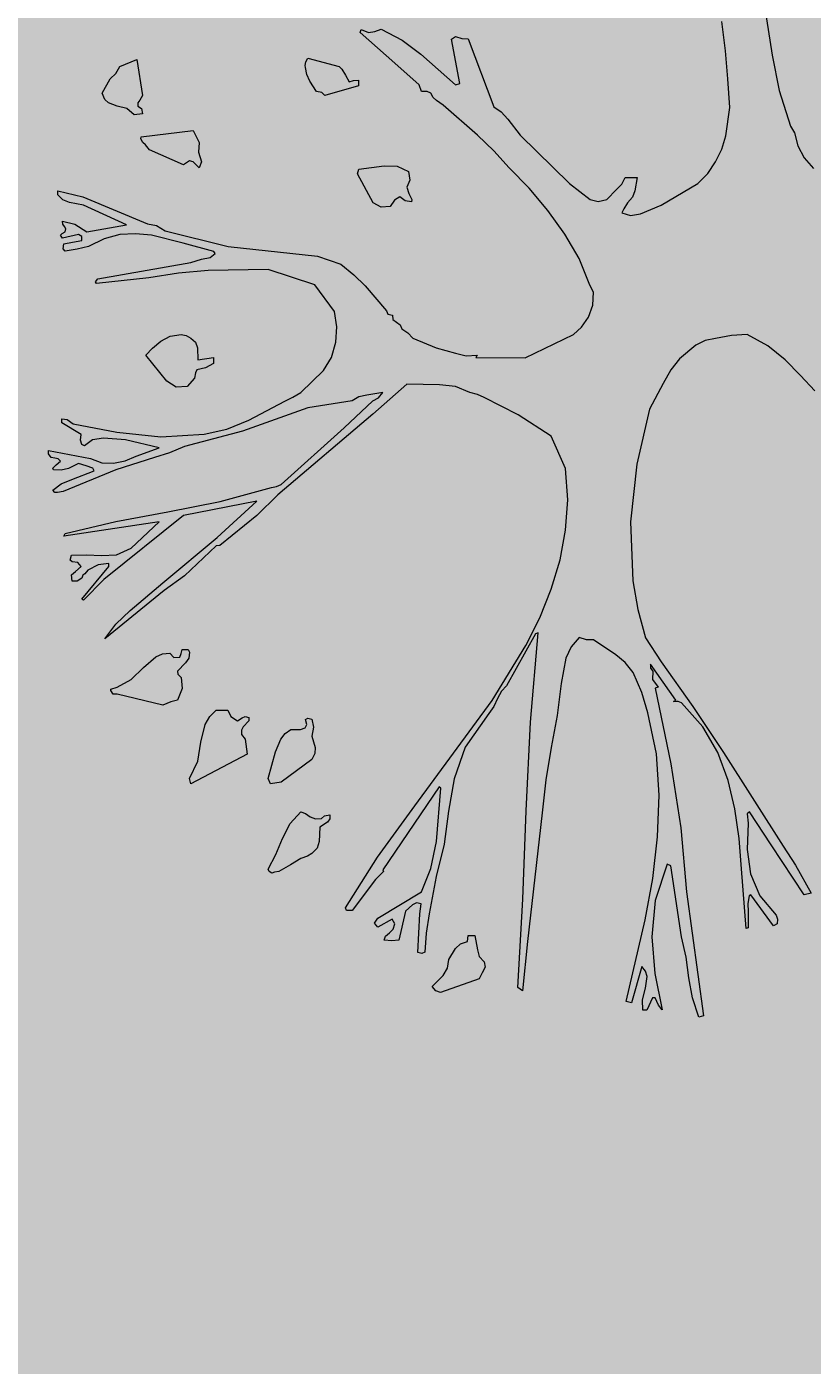
# Model space of a CAD drawing. Units: inches. Extents: x 84 to 1044, y -280 to 906.
# Tile 57 of 105: x 387.99 to 401.24, y 738.5 to 761.07. Entities that reach past the tile are written whole.
import ezdxf

# ---------------------------------------------------------------- set-up
doc = ezdxf.new("R2010")
doc.units = ezdxf.units.IN
doc.layers.add('A-ANNO-DIMS', color=2, linetype='Continuous', lineweight=18)
doc.layers.add('L-PLNT', color=114, linetype='Continuous', lineweight=15)
doc.layers.add('L-PLNT-PATT', color=9, linetype='Continuous', lineweight=9, true_color=0xafd9aa)
doc.styles.get("Standard").update_dxf_attribs({"font": 'arial.ttf'})
doc.dimstyles.get("Standard").update_dxf_attribs({"dimtxt": 0.18, "dimasz": 0.18, "dimexe": 0.18, "dimexo": 0.0625, "dimgap": 0.09, "dimtad": 0, "dimtih": 1, "dimtoh": 1, "dimdec": 4, "dimzin": 0, "dimdsep": 46, "dimtxsty": 'Standard', "dimcen": 0.09, "dimadec": 0, "dimazin": 0, "dimtfac": 1, "dimtdec": 4, "dimtofl": 0, "dimtmove": 0, "dimatfit": 3, "dimfxl": 1, "dimtolj": 1, "dimtzin": 0, "dimarcsym": 0})

# ---------------------------------------------------------------- blocks, each defined once
blk = doc.blocks.new('A$C37E508DF')
for p, q in [((0.7911, 1.1436), (0.8027, 1.0677)), ((0.7512, 1.0728), (0.7469, 1.1054)), ((0.3456, 1.093), (0.3469, 1.0964)), ((0.3842, 1.0591), (0.3456, 1.093)), ((0.3469, 1.0964), (0.355, 1.093)), ((0.355, 1.093), (0.3619, 1.0943)), ((0.3619, 1.0943), (0.3692, 1.0968)), ((0.3692, 1.0968), (0.3923, 1.0844)), ((0.4472, 1.0857), (0.4515, 1.0887)), ((0.4562, 1.0364), (0.4472, 1.0857)), ((0.4515, 1.0887), (0.4584, 1.0865)), ((0.4584, 1.0865), (0.4657, 1.0861)), ((0.4657, 1.0861), (0.4939, 1.0107)), ((0.3923, 1.0844), (0.4129, 1.069)), ((0.7538, 1.0415), (0.7512, 1.0728)), ((0.0746, 1.0475), (0.0789, 1.0552)), ((0.0789, 1.0552), (0.0978, 1.063)), ((0.0978, 1.063), (0.1042, 1.0231)), ((0.2847, 1.0565), (0.2856, 1.0604)), ((0.2851, 1.054), (0.2847, 1.0565)), ((0.2856, 1.0604), (0.2877, 1.0647)), ((0.2877, 1.0647), (0.3224, 1.0552)), ((0.3224, 1.0552), (0.3255, 1.0522)), ((0.4112, 1.0351), (0.3842, 1.0591)), ((0.4129, 1.069), (0.4515, 1.0351)), ((0.8027, 1.0677), (0.8108, 1.0287)), ((0.0596, 1.0257), (0.0682, 1.0415)), ((0.0682, 1.0415), (0.0746, 1.0475)), ((0.2864, 1.0463), (0.2851, 1.054)), ((0.2899, 1.039), (0.2864, 1.0463)), ((0.3255, 1.0522), (0.3293, 1.0458)), ((0.3293, 1.0458), (0.3336, 1.0381)), ((0.3383, 1.0398), (0.3439, 1.0402)), ((0.3439, 1.0402), (0.3439, 1.0338)), ((0.7559, 1.0098), (0.7538, 1.0415)), ((0.0626, 1.0188), (0.0596, 1.0257)), ((0.2972, 1.0274), (0.2899, 1.039)), ((0.3032, 1.0265), (0.2972, 1.0274)), ((0.3066, 1.0231), (0.3032, 1.0265)), ((0.3439, 1.0338), (0.3066, 1.0231)), ((0.3336, 1.0381), (0.3383, 1.0398)), ((0.4138, 1.0274), (0.4112, 1.0351)), ((0.4202, 1.0274), (0.4138, 1.0274)), ((0.4241, 1.0257), (0.4202, 1.0274)), ((0.4267, 1.0209), (0.4241, 1.0257)), ((0.4515, 1.0351), (0.4562, 1.0364)), ((0.8108, 1.0287), (0.8233, 0.9892)), ((0.0665, 1.0149), (0.0626, 1.0188)), ((0.0763, 1.0111), (0.0665, 1.0149)), ((0.087, 1.0085), (0.0763, 1.0111)), ((0.1012, 1.018), (0.099, 1.0149)), ((0.099, 1.0149), (0.099, 1.0111)), ((0.099, 1.0111), (0.1033, 1.0085)), ((0.1042, 1.0231), (0.1012, 1.018)), ((0.4305, 1.0175), (0.4267, 1.0209)), ((0.4378, 1.0124), (0.4305, 1.0175)), ((0.476, 0.9789), (0.4378, 1.0124)), ((0.4939, 1.0107), (0.5021, 1.0051)), ((0.0948, 1.0016), (0.087, 1.0085)), ((0.1042, 1.0029), (0.0948, 1.0016)), ((0.1033, 1.0085), (0.1042, 1.0029)), ((0.5021, 1.0051), (0.5094, 0.9969)), ((0.5094, 0.9969), (0.5231, 0.9789)), ((0.7516, 0.9785), (0.7559, 1.0098)), ((0.1029, 0.9772), (0.1604, 0.9841)), ((0.1604, 0.9841), (0.1672, 0.9708)), ((0.8233, 0.9892), (0.8275, 0.9815)), ((0.8275, 0.9815), (0.8314, 0.9673)), ((0.1025, 0.9751), (0.1029, 0.9772)), ((0.1046, 0.9708), (0.1025, 0.9751)), ((0.1076, 0.9682), (0.1046, 0.9708)), ((0.1119, 0.9626), (0.1076, 0.9682)), ((0.1672, 0.9708), (0.1664, 0.9601)), ((0.4939, 0.9618), (0.476, 0.9789)), ((0.5231, 0.9789), (0.578, 0.9253)), ((0.7469, 0.9635), (0.7516, 0.9785)), ((0.8314, 0.9673), (0.8383, 0.954)), ((0.1496, 0.9463), (0.1119, 0.9626)), ((0.1664, 0.9601), (0.1698, 0.9493)), ((0.5111, 0.9429), (0.4939, 0.9618)), ((0.7401, 0.9493), (0.7469, 0.9635)), ((0.8383, 0.954), (0.8486, 0.942)), ((0.1565, 0.9506), (0.1496, 0.9463)), ((0.1604, 0.9493), (0.1565, 0.9506)), ((0.1629, 0.9468), (0.1604, 0.9493)), ((0.1672, 0.9429), (0.1629, 0.9468)), ((0.1698, 0.9493), (0.1672, 0.9429)), ((0.3426, 0.936), (0.3443, 0.9412)), ((0.3443, 0.9412), (0.3722, 0.9451)), ((0.3722, 0.9451), (0.3868, 0.9446)), ((0.3868, 0.9446), (0.3992, 0.9386)), ((0.3992, 0.9386), (0.4009, 0.9292)), ((0.5334, 0.9202), (0.5111, 0.9429)), ((0.7203, 0.9253), (0.7315, 0.9365)), ((0.7315, 0.9365), (0.7401, 0.9493)), ((0.3602, 0.9039), (0.3426, 0.936)), ((0.4009, 0.9292), (0.3975, 0.9215)), ((0.3975, 0.9215), (0.3996, 0.9142)), ((0.578, 0.9253), (0.6011, 0.9077)), ((0.6303, 0.9189), (0.6359, 0.9245)), ((0.6359, 0.9245), (0.6397, 0.9322)), ((0.6397, 0.9322), (0.653, 0.9322)), ((0.653, 0.9322), (0.6505, 0.9172)), ((0.6796, 0.9013), (0.7203, 0.9253)), ((0.0103, 0.9129), (0.0103, 0.9172)), ((0.0103, 0.9172), (0.0382, 0.9107)), ((0.0159, 0.9073), (0.0103, 0.9129)), ((0.0232, 0.9043), (0.0159, 0.9073)), ((0.0382, 0.9107), (0.1098, 0.8807)), ((0.3838, 0.9069), (0.379, 0.9)), ((0.3898, 0.9107), (0.3838, 0.9069)), ((0.3958, 0.906), (0.3898, 0.9107)), ((0.3996, 0.9142), (0.4031, 0.9077)), ((0.4031, 0.9077), (0.4026, 0.9052)), ((0.554, 0.8953), (0.5334, 0.9202)), ((0.6011, 0.9077), (0.6097, 0.9056)), ((0.6097, 0.9056), (0.6196, 0.9077)), ((0.6196, 0.9077), (0.6303, 0.9189)), ((0.6479, 0.9103), (0.6423, 0.9039)), ((0.6505, 0.9172), (0.6479, 0.9103)), ((0.0386, 0.9013), (0.0232, 0.9043)), ((0.0866, 0.8794), (0.0386, 0.9013)), ((0.3692, 0.8992), (0.3602, 0.9039)), ((0.379, 0.9), (0.3692, 0.8992)), ((0.4026, 0.9052), (0.3958, 0.906)), ((0.5728, 0.8691), (0.554, 0.8953)), ((0.6384, 0.8974), (0.6359, 0.8927)), ((0.6359, 0.8927), (0.6457, 0.8897)), ((0.6423, 0.9039), (0.6384, 0.8974)), ((0.6457, 0.8897), (0.6569, 0.8919)), ((0.6569, 0.8919), (0.6796, 0.9013)), ((0.0159, 0.8803), (0.0154, 0.8837)), ((0.0154, 0.8837), (0.0292, 0.8803)), ((0.0176, 0.8777), (0.0159, 0.8803)), ((0.0193, 0.8752), (0.0176, 0.8777)), ((0.0292, 0.8803), (0.0424, 0.8717)), ((0.0424, 0.8717), (0.0866, 0.8794)), ((0.1098, 0.8807), (0.1196, 0.8786)), ((0.1196, 0.8786), (0.1295, 0.873)), ((0.0133, 0.8679), (0.015, 0.87)), ((0.0154, 0.8649), (0.0133, 0.8679)), ((0.015, 0.87), (0.0184, 0.8717)), ((0.0334, 0.8687), (0.0154, 0.8649)), ((0.0184, 0.8717), (0.0193, 0.8752)), ((0.0266, 0.8602), (0.0369, 0.8623)), ((0.0369, 0.8666), (0.0334, 0.8687)), ((0.0369, 0.8623), (0.0369, 0.8666)), ((0.0617, 0.864), (0.0442, 0.8554)), ((0.0789, 0.8687), (0.0617, 0.864)), ((0.0965, 0.8696), (0.0789, 0.8687)), ((0.1141, 0.8679), (0.0965, 0.8696)), ((0.1492, 0.8593), (0.1141, 0.8679)), ((0.1295, 0.873), (0.1994, 0.8554)), ((0.5887, 0.8421), (0.5728, 0.8691)), ((0.0163, 0.8529), (0.0171, 0.8584)), ((0.0184, 0.8503), (0.0163, 0.8529)), ((0.0171, 0.8584), (0.0266, 0.8602)), ((0.0317, 0.8524), (0.0184, 0.8503)), ((0.0442, 0.8554), (0.0317, 0.8524)), ((0.1835, 0.8499), (0.1492, 0.8593)), ((0.1792, 0.8434), (0.1848, 0.8477)), ((0.1848, 0.8477), (0.1835, 0.8499)), ((0.1994, 0.8554), (0.2984, 0.8447)), ((0.0545, 0.8194), (0.1578, 0.8378)), ((0.1578, 0.8378), (0.1698, 0.8413)), ((0.1698, 0.8413), (0.1792, 0.8434)), ((0.2984, 0.8447), (0.3242, 0.8357)), ((0.3242, 0.8357), (0.3387, 0.8241)), ((0.6007, 0.8125), (0.5887, 0.8421)), ((0.0519, 0.8164), (0.0545, 0.8194)), ((0.1111, 0.8207), (0.0532, 0.8143)), ((0.1441, 0.8258), (0.1111, 0.8207)), ((0.1771, 0.8288), (0.1441, 0.8258)), ((0.2436, 0.8301), (0.1771, 0.8288)), ((0.2954, 0.813), (0.2436, 0.8301)), ((0.3387, 0.8241), (0.3512, 0.8117)), ((0.0532, 0.8143), (0.0519, 0.8164)), ((0.3173, 0.7834), (0.2954, 0.813)), ((0.3512, 0.8117), (0.3748, 0.7842)), ((0.6046, 0.8048), (0.6007, 0.8125)), ((0.6037, 0.7903), (0.6046, 0.8048)), ((0.599, 0.777), (0.6037, 0.7903)), ((0.3199, 0.7662), (0.3173, 0.7834)), ((0.3748, 0.7842), (0.3765, 0.7804)), ((0.3765, 0.7804), (0.3816, 0.7791)), ((0.3816, 0.7791), (0.382, 0.7744)), ((0.382, 0.7744), (0.3859, 0.7714)), ((0.5913, 0.7658), (0.599, 0.777)), ((0.3186, 0.7491), (0.3199, 0.7662)), ((0.3859, 0.7714), (0.3902, 0.7684)), ((0.3902, 0.7684), (0.3919, 0.7641)), ((0.3919, 0.7641), (0.3988, 0.7598)), ((0.3988, 0.7598), (0.4043, 0.7538)), ((0.5823, 0.7577), (0.5913, 0.7658)), ((0.1153, 0.7427), (0.1244, 0.7504)), ((0.1244, 0.7504), (0.1351, 0.7559)), ((0.1351, 0.7559), (0.1471, 0.7577)), ((0.1471, 0.7577), (0.1527, 0.7568)), ((0.1527, 0.7568), (0.1578, 0.7538)), ((0.1578, 0.7538), (0.1629, 0.7491)), ((0.1629, 0.7491), (0.1651, 0.7431)), ((0.1651, 0.7431), (0.1655, 0.7298)), ((0.3139, 0.7324), (0.3186, 0.7491)), ((0.4043, 0.7538), (0.4301, 0.7431)), ((0.4301, 0.7431), (0.4515, 0.7371)), ((0.5287, 0.7319), (0.5823, 0.7577)), ((0.7182, 0.7461), (0.7002, 0.7307)), ((0.7285, 0.7512), (0.7182, 0.7461)), ((0.7401, 0.7534), (0.7285, 0.7512)), ((0.7577, 0.7568), (0.7401, 0.7534)), ((0.7752, 0.7577), (0.7577, 0.7568)), ((0.798, 0.7452), (0.7752, 0.7577)), ((0.8173, 0.7298), (0.798, 0.7452)), ((0.1081, 0.7349), (0.1153, 0.7427)), ((0.1312, 0.7058), (0.1081, 0.7349)), ((0.1655, 0.7298), (0.1831, 0.7324)), ((0.1831, 0.7324), (0.1831, 0.7255)), ((0.3049, 0.7178), (0.3139, 0.7324)), ((0.4515, 0.7371), (0.4635, 0.7341)), ((0.4635, 0.7341), (0.4755, 0.7349)), ((0.4755, 0.7349), (0.4742, 0.7324)), ((0.4742, 0.7324), (0.5287, 0.7319)), ((0.7002, 0.7307), (0.6903, 0.7186)), ((0.8344, 0.7122), (0.8173, 0.7298)), ((0.1629, 0.7152), (0.1621, 0.7092)), ((0.1646, 0.7186), (0.1629, 0.7152)), ((0.1741, 0.7208), (0.1646, 0.7186)), ((0.1831, 0.7255), (0.1741, 0.7208)), ((0.28, 0.6933), (0.3049, 0.7178)), ((0.6903, 0.7186), (0.6818, 0.7032)), ((0.1415, 0.6994), (0.1312, 0.7058)), ((0.1539, 0.7002), (0.1415, 0.6994)), ((0.1621, 0.7092), (0.1539, 0.7002)), ((0.3975, 0.7028), (0.3598, 0.6693)), ((0.4339, 0.7019), (0.3975, 0.7028)), ((0.4515, 0.7002), (0.4339, 0.7019)), ((0.4674, 0.6933), (0.4515, 0.7002)), ((0.6818, 0.7032), (0.6667, 0.6749)), ((0.8503, 0.6951), (0.8344, 0.7122)), ((0.2221, 0.6625), (0.262, 0.6839)), ((0.262, 0.6839), (0.271, 0.6882)), ((0.271, 0.6882), (0.28, 0.6933)), ((0.337, 0.6843), (0.2877, 0.6762)), ((0.328, 0.6543), (0.3598, 0.6843)), ((0.3443, 0.6886), (0.337, 0.6843)), ((0.3533, 0.6903), (0.3443, 0.6886)), ((0.3709, 0.6933), (0.3533, 0.6903)), ((0.3598, 0.6843), (0.3662, 0.6873)), ((0.3662, 0.6873), (0.3709, 0.6933)), ((0.476, 0.6912), (0.4674, 0.6933)), ((0.4832, 0.6878), (0.476, 0.6912)), ((0.521, 0.6685), (0.4832, 0.6878)), ((0.2877, 0.6762), (0.2152, 0.6505)), ((0.3598, 0.6693), (0.2543, 0.5797)), ((0.6667, 0.6749), (0.6526, 0.614)), ((0.0146, 0.6599), (0.0146, 0.6642)), ((0.0146, 0.6642), (0.0206, 0.6633)), ((0.036, 0.6466), (0.0146, 0.6599)), ((0.0206, 0.6633), (0.0274, 0.6586)), ((0.0274, 0.6586), (0.0759, 0.6492)), ((0.1977, 0.6526), (0.2221, 0.6625)), ((0.2581, 0.5913), (0.328, 0.6543)), ((0.5578, 0.6449), (0.521, 0.6685)), ((0.0356, 0.6406), (0.036, 0.6466)), ((0.0369, 0.6355), (0.0356, 0.6406)), ((0.0489, 0.641), (0.0399, 0.6342)), ((0.0609, 0.6428), (0.0489, 0.641)), ((0.0853, 0.641), (0.0609, 0.6428)), ((0.0759, 0.6492), (0.1244, 0.644)), ((0.1226, 0.632), (0.0853, 0.641)), ((0.1244, 0.644), (0.1728, 0.647)), ((0.2152, 0.6505), (0.1509, 0.6333)), ((0.1728, 0.647), (0.1977, 0.6526)), ((0.5737, 0.6089), (0.5578, 0.6449)), ((0, 0.629), (0.0467, 0.62)), ((0, 0.6252), (0, 0.629)), ((0.003, 0.6213), (0, 0.6252)), ((0.0399, 0.6342), (0.0369, 0.6355)), ((0.0973, 0.6226), (0.1226, 0.632)), ((0.1342, 0.6265), (0.1175, 0.6213)), ((0.1509, 0.6333), (0.1342, 0.6265)), ((0.0069, 0.6204), (0.003, 0.6213)), ((0.0047, 0.6093), (0.0086, 0.6132)), ((0.0056, 0.6076), (0.0047, 0.6093)), ((0.0107, 0.6196), (0.0069, 0.6204)), ((0.0086, 0.6132), (0.0133, 0.617)), ((0.0133, 0.617), (0.0107, 0.6196)), ((0.0334, 0.6145), (0.0223, 0.6089)), ((0.0416, 0.6119), (0.0334, 0.6145)), ((0.0493, 0.6093), (0.0416, 0.6119)), ((0.0467, 0.62), (0.0592, 0.6153)), ((0.0506, 0.6063), (0.0493, 0.6093)), ((0.0592, 0.6153), (0.072, 0.6149)), ((0.072, 0.6149), (0.0849, 0.6175)), ((0.1175, 0.6213), (0.0746, 0.6076)), ((0.0849, 0.6175), (0.0973, 0.6226)), ((0.6526, 0.614), (0.6457, 0.5497)), ((0.0141, 0.6072), (0.0056, 0.6076)), ((0.0223, 0.6089), (0.0141, 0.6072)), ((0.0141, 0.5921), (0.0257, 0.5969)), ((0.0746, 0.6076), (0.0163, 0.5836)), ((0.0257, 0.5969), (0.0506, 0.6063)), ((0.5763, 0.5741), (0.5737, 0.6089)), ((0.0047, 0.5849), (0.0141, 0.5921)), ((0.0069, 0.5823), (0.0047, 0.5849)), ((0.0099, 0.5823), (0.0069, 0.5823)), ((0.0163, 0.5836), (0.0099, 0.5823)), ((0.1904, 0.5724), (0.2474, 0.5879)), ((0.2543, 0.5797), (0.2311, 0.557)), ((0.2474, 0.5879), (0.253, 0.5892)), ((0.253, 0.5892), (0.2581, 0.5913)), ((0.1325, 0.5608), (0.1904, 0.5724)), ((0.2311, 0.5729), (0.1496, 0.557)), ((0.1869, 0.5325), (0.2311, 0.5729)), ((0.5737, 0.5407), (0.5763, 0.5741)), ((0.0184, 0.5368), (0.0746, 0.5501)), ((0.1496, 0.557), (0.0613, 0.4858)), ((0.0746, 0.5501), (0.1325, 0.5608)), ((0.2311, 0.557), (0.1899, 0.5235)), ((0.1226, 0.5497), (0.0171, 0.5338)), ((0.0171, 0.5338), (0.0184, 0.5368)), ((0.0917, 0.5205), (0.1226, 0.5497)), ((0.5677, 0.5077), (0.5737, 0.5407)), ((0.6457, 0.5497), (0.6483, 0.4845)), ((0.0755, 0.5133), (0.0917, 0.5205)), ((0.1269, 0.482), (0.1869, 0.5325)), ((0.1861, 0.5231), (0.1509, 0.4897)), ((0.1899, 0.5235), (0.1861, 0.5231)), ((0.024, 0.5072), (0.0253, 0.5128)), ((0.0262, 0.5055), (0.024, 0.5072)), ((0.0253, 0.5128), (0.042, 0.5133)), ((0.0326, 0.5047), (0.0262, 0.5055)), ((0.042, 0.5133), (0.0587, 0.5124)), ((0.0587, 0.5124), (0.0755, 0.5133)), ((0.5578, 0.4751), (0.5677, 0.5077)), ((0.0253, 0.491), (0.03, 0.4948)), ((0.0262, 0.4841), (0.0253, 0.491)), ((0.03, 0.4948), (0.036, 0.5004)), ((0.036, 0.5004), (0.0326, 0.5047)), ((0.0369, 0.4639), (0.0669, 0.5004)), ((0.0382, 0.4905), (0.0369, 0.4871)), ((0.0403, 0.4922), (0.0382, 0.4905)), ((0.0437, 0.4961), (0.0403, 0.4922)), ((0.0549, 0.5021), (0.0437, 0.4961)), ((0.0669, 0.5034), (0.0549, 0.5021)), ((0.0669, 0.5004), (0.0669, 0.5034)), ((0.0317, 0.4841), (0.0262, 0.4841)), ((0.0369, 0.4871), (0.0317, 0.4841)), ((0.0613, 0.4858), (0.0386, 0.4627)), ((0.0905, 0.4515), (0.1269, 0.482)), ((0.1509, 0.4897), (0.1282, 0.4734)), ((0.6483, 0.4845), (0.6539, 0.4524)), ((0.0386, 0.4627), (0.0369, 0.4639)), ((0.1282, 0.4734), (0.0626, 0.4198)), ((0.545, 0.4434), (0.5578, 0.4751)), ((0.0746, 0.4361), (0.0905, 0.4515)), ((0.6539, 0.4524), (0.6625, 0.4211)), ((0.0626, 0.4198), (0.0746, 0.4361)), ((0.5295, 0.4125), (0.545, 0.4434)), ((0.5403, 0.4254), (0.5081, 0.3679)), ((0.5347, 0.3276), (0.5433, 0.4266)), ((0.5433, 0.4266), (0.5403, 0.4254)), ((0.5887, 0.4215), (0.5797, 0.4112)), ((0.5969, 0.4189), (0.5887, 0.4215)), ((0.6046, 0.4189), (0.5969, 0.4189)), ((0.6295, 0.4022), (0.6046, 0.4189)), ((0.6625, 0.4211), (0.6796, 0.3945)), ((0.1192, 0.4001), (0.1265, 0.4031)), ((0.1265, 0.4031), (0.1346, 0.4039)), ((0.1346, 0.4039), (0.1389, 0.3992)), ((0.1458, 0.3996), (0.1471, 0.4035)), ((0.1471, 0.4035), (0.1484, 0.4082)), ((0.1484, 0.4082), (0.1548, 0.4082)), ((0.1548, 0.4082), (0.1565, 0.4052)), ((0.1565, 0.4052), (0.1556, 0.3983)), ((0.4922, 0.3516), (0.5295, 0.4125)), ((0.5797, 0.4112), (0.5741, 0.3983)), ((0.6397, 0.3936), (0.6295, 0.4022)), ((0.0917, 0.3748), (0.1055, 0.388)), ((0.1055, 0.388), (0.1192, 0.4001)), ((0.1389, 0.3992), (0.1458, 0.3996)), ((0.1518, 0.3932), (0.1432, 0.3842)), ((0.1556, 0.3983), (0.1518, 0.3932)), ((0.5741, 0.3983), (0.5686, 0.3705)), ((0.6487, 0.3825), (0.6397, 0.3936)), ((0.6959, 0.352), (0.668, 0.3919)), ((0.668, 0.3919), (0.668, 0.3872)), ((0.668, 0.3872), (0.6706, 0.3842)), ((0.6796, 0.3945), (0.7148, 0.3447)), ((0.0763, 0.3662), (0.0917, 0.3748)), ((0.1432, 0.3842), (0.1436, 0.3808)), ((0.1436, 0.3808), (0.1471, 0.3769)), ((0.1471, 0.3769), (0.1484, 0.3649)), ((0.6582, 0.3602), (0.6487, 0.3825)), ((0.6706, 0.3842), (0.6702, 0.3748)), ((0.6702, 0.3748), (0.6762, 0.3662)), ((0.069, 0.364), (0.0763, 0.3662)), ((0.069, 0.3627), (0.069, 0.364)), ((0.0716, 0.3585), (0.069, 0.3627)), ((0.0763, 0.3585), (0.0716, 0.3585)), ((0.1269, 0.3464), (0.0763, 0.3585)), ((0.1484, 0.3649), (0.1432, 0.352)), ((0.5025, 0.3619), (0.4982, 0.3537)), ((0.5081, 0.3679), (0.5025, 0.3619)), ((0.5686, 0.3705), (0.5643, 0.3349)), ((0.665, 0.3379), (0.6582, 0.3602)), ((0.6762, 0.3662), (0.6732, 0.3653)), ((0.6732, 0.3653), (0.6903, 0.2813)), ((0.1355, 0.3499), (0.1269, 0.3464)), ((0.1432, 0.352), (0.1355, 0.3499)), ((0.4065, 0.2345), (0.4922, 0.3516)), ((0.4939, 0.3447), (0.4884, 0.337)), ((0.4982, 0.3537), (0.4939, 0.3447)), ((0.6933, 0.3503), (0.6959, 0.352)), ((0.6985, 0.3503), (0.6933, 0.3503)), ((0.7023, 0.349), (0.6985, 0.3503)), ((0.7259, 0.3224), (0.7023, 0.349)), ((0.7148, 0.3447), (0.7487, 0.2937)), ((0.1737, 0.325), (0.1788, 0.3336)), ((0.1788, 0.3336), (0.1861, 0.3409)), ((0.1861, 0.3409), (0.199, 0.3409)), ((0.199, 0.3409), (0.2024, 0.3336)), ((0.2024, 0.3336), (0.2097, 0.3289)), ((0.2097, 0.3289), (0.2148, 0.3323)), ((0.2148, 0.3323), (0.2182, 0.3336)), ((0.2221, 0.3289), (0.2161, 0.3224)), ((0.2182, 0.3336), (0.2221, 0.3327)), ((0.2221, 0.3327), (0.2221, 0.3289)), ((0.2851, 0.3302), (0.2877, 0.3319)), ((0.2864, 0.325), (0.2851, 0.3302)), ((0.2877, 0.3319), (0.292, 0.3306)), ((0.292, 0.3306), (0.2941, 0.322)), ((0.4884, 0.337), (0.4622, 0.2997)), ((0.53, 0.229), (0.5347, 0.3276)), ((0.5643, 0.3349), (0.5578, 0.2993)), ((0.6745, 0.2924), (0.665, 0.3379)), ((0.1689, 0.3053), (0.1737, 0.325)), ((0.2161, 0.3224), (0.214, 0.3186)), ((0.214, 0.3186), (0.214, 0.3139)), ((0.214, 0.3139), (0.2182, 0.3087)), ((0.2577, 0.3087), (0.2624, 0.3147)), ((0.2624, 0.3147), (0.2689, 0.3194)), ((0.2689, 0.3194), (0.2796, 0.3194)), ((0.2796, 0.3194), (0.2847, 0.3211)), ((0.2847, 0.3211), (0.2864, 0.325)), ((0.2941, 0.322), (0.292, 0.3117)), ((0.7427, 0.2937), (0.7259, 0.3224)), ((0.1655, 0.2843), (0.1689, 0.3053)), ((0.2182, 0.3087), (0.2204, 0.292)), ((0.2517, 0.2946), (0.2577, 0.3087)), ((0.292, 0.3117), (0.2959, 0.2993)), ((0.2959, 0.2993), (0.2954, 0.2928)), ((0.4622, 0.2997), (0.4502, 0.2645)), ((0.5578, 0.2993), (0.5518, 0.2633)), ((0.1565, 0.265), (0.1655, 0.2843)), ((0.2204, 0.292), (0.1578, 0.259)), ((0.2436, 0.265), (0.2517, 0.2946)), ((0.292, 0.286), (0.2581, 0.2607)), ((0.2954, 0.2928), (0.292, 0.286)), ((0.6775, 0.2465), (0.6745, 0.2924)), ((0.7542, 0.2628), (0.7427, 0.2937)), ((0.7487, 0.2937), (0.8151, 0.1899)), ((0.6903, 0.2813), (0.7015, 0.2101)), ((0.1578, 0.259), (0.1565, 0.265)), ((0.2461, 0.259), (0.2436, 0.265)), ((0.2581, 0.2607), (0.2461, 0.259)), ((0.4335, 0.2556), (0.3709, 0.1634)), ((0.4305, 0.1951), (0.4352, 0.2543)), ((0.4352, 0.2543), (0.4335, 0.2556)), ((0.4502, 0.2645), (0.4438, 0.2285)), ((0.5518, 0.2633), (0.5475, 0.2268)), ((0.7615, 0.2311), (0.7542, 0.2628)), ((0.6758, 0.2002), (0.6775, 0.2465)), ((0.268, 0.2148), (0.28, 0.2277)), ((0.28, 0.2277), (0.2851, 0.226)), ((0.2851, 0.226), (0.2903, 0.2225)), ((0.3027, 0.2204), (0.3061, 0.2234)), ((0.3061, 0.2234), (0.3122, 0.2247)), ((0.3122, 0.2247), (0.3122, 0.22)), ((0.3649, 0.1775), (0.4065, 0.2345)), ((0.4438, 0.2285), (0.4391, 0.1921)), ((0.5261, 0.1308), (0.53, 0.229)), ((0.5475, 0.2268), (0.5313, 0.084)), ((0.7662, 0.1981), (0.7615, 0.2311)), ((0.7778, 0.2277), (0.7752, 0.2255)), ((0.7752, 0.2255), (0.7761, 0.2152)), ((0.8018, 0.1912), (0.7778, 0.2277)), ((0.2594, 0.1981), (0.268, 0.2148)), ((0.2903, 0.2225), (0.2963, 0.22)), ((0.2963, 0.22), (0.3027, 0.2204)), ((0.301, 0.211), (0.3002, 0.1951)), ((0.3096, 0.2165), (0.301, 0.211)), ((0.3122, 0.22), (0.3096, 0.2165)), ((0.7015, 0.2101), (0.7079, 0.1389)), ((0.7761, 0.2152), (0.7752, 0.1861)), ((0.2521, 0.1805), (0.2594, 0.1981)), ((0.3002, 0.1951), (0.298, 0.1874)), ((0.4241, 0.1651), (0.4305, 0.1951)), ((0.6706, 0.1539), (0.6758, 0.2002)), ((0.7688, 0.1646), (0.7662, 0.1981)), ((0.2436, 0.1642), (0.2521, 0.1805)), ((0.2873, 0.1788), (0.28, 0.1762)), ((0.292, 0.1818), (0.2873, 0.1788)), ((0.298, 0.1874), (0.292, 0.1818)), ((0.4391, 0.1921), (0.4301, 0.1561)), ((0.7752, 0.1861), (0.7787, 0.1591)), ((0.8383, 0.1359), (0.8018, 0.1912)), ((0.8151, 0.1899), (0.8288, 0.1685)), ((0.2448, 0.1616), (0.2436, 0.1642)), ((0.2684, 0.1689), (0.2556, 0.1616)), ((0.28, 0.1762), (0.2684, 0.1689)), ((0.3293, 0.1213), (0.3649, 0.1775)), ((0.4138, 0.1389), (0.4241, 0.1651)), ((0.6865, 0.1698), (0.6732, 0.1295)), ((0.6903, 0.1681), (0.6865, 0.1698)), ((0.7023, 0.0892), (0.6903, 0.1681)), ((0.774, 0.0982), (0.7688, 0.1646)), ((0.8288, 0.1685), (0.846, 0.1376)), ((0.2478, 0.1599), (0.2448, 0.1616)), ((0.2508, 0.1608), (0.2478, 0.1599)), ((0.2556, 0.1616), (0.2508, 0.1608)), ((0.3628, 0.1526), (0.337, 0.1183)), ((0.3692, 0.1591), (0.3628, 0.1526)), ((0.3718, 0.1616), (0.3692, 0.1591)), ((0.3709, 0.1634), (0.3718, 0.1616)), ((0.4301, 0.1561), (0.4224, 0.1145)), ((0.662, 0.108), (0.6706, 0.1539)), ((0.7787, 0.1591), (0.789, 0.1346)), ((0.3653, 0.1098), (0.4138, 0.1389)), ((0.7079, 0.1389), (0.7268, 0.0013)), ((0.7774, 0.1346), (0.7757, 0.1261)), ((0.7791, 0.1359), (0.7774, 0.1346)), ((0.8044, 0.1012), (0.7791, 0.1359)), ((0.789, 0.1346), (0.8074, 0.1132)), ((0.846, 0.1376), (0.8383, 0.1359)), ((0.3306, 0.1183), (0.3293, 0.1213)), ((0.4039, 0.1248), (0.3962, 0.1175)), ((0.4082, 0.1269), (0.4039, 0.1248)), ((0.4134, 0.1256), (0.4082, 0.1269)), ((0.4121, 0.1145), (0.4134, 0.1256)), ((0.5205, 0.033), (0.5261, 0.1308)), ((0.6732, 0.1295), (0.6693, 0.0892)), ((0.7757, 0.1261), (0.7761, 0.117)), ((0.337, 0.1183), (0.3306, 0.1183)), ((0.3615, 0.1042), (0.3653, 0.1098)), ((0.3653, 0.0999), (0.3615, 0.1042)), ((0.3812, 0.1089), (0.3653, 0.0999)), ((0.3842, 0.1037), (0.3812, 0.1089)), ((0.3962, 0.1175), (0.3885, 0.0853)), ((0.4099, 0.0716), (0.4121, 0.1145)), ((0.4224, 0.1145), (0.4189, 0.093)), ((0.641, 0.0172), (0.662, 0.108)), ((0.7761, 0.117), (0.7761, 0.099)), ((0.8074, 0.1132), (0.8087, 0.1089)), ((0.8087, 0.1089), (0.8083, 0.1037)), ((0.3722, 0.0853), (0.3739, 0.09)), ((0.3739, 0.09), (0.3782, 0.0935)), ((0.3782, 0.0935), (0.3825, 0.0978)), ((0.3825, 0.0978), (0.3842, 0.1037)), ((0.4189, 0.093), (0.4176, 0.072)), ((0.4648, 0.084), (0.4657, 0.0905)), ((0.4657, 0.0905), (0.473, 0.0905)), ((0.473, 0.0905), (0.476, 0.0746)), ((0.6693, 0.0892), (0.6728, 0.0484)), ((0.7075, 0.0665), (0.7023, 0.0892)), ((0.7761, 0.099), (0.774, 0.0982)), ((0.8083, 0.1037), (0.8044, 0.1012)), ((0.3808, 0.0845), (0.3722, 0.0853)), ((0.3885, 0.0853), (0.3808, 0.0845)), ((0.4442, 0.0639), (0.4515, 0.0763)), ((0.4515, 0.0763), (0.4571, 0.0815)), ((0.4571, 0.0815), (0.4648, 0.084)), ((0.476, 0.0746), (0.4777, 0.0673)), ((0.5313, 0.084), (0.5257, 0.0291)), ((0.4142, 0.0707), (0.4099, 0.0716)), ((0.4176, 0.072), (0.4142, 0.0707)), ((0.4425, 0.0544), (0.4442, 0.0639)), ((0.4777, 0.0673), (0.4832, 0.0613)), ((0.4832, 0.0613), (0.4845, 0.0553)), ((0.7105, 0.0437), (0.7075, 0.0665)), ((0.4258, 0.0339), (0.4378, 0.0463)), ((0.4378, 0.0463), (0.4425, 0.0544)), ((0.4811, 0.0493), (0.4777, 0.0424)), ((0.4845, 0.0553), (0.4811, 0.0493)), ((0.6582, 0.0562), (0.6466, 0.0159)), ((0.6625, 0.051), (0.6582, 0.0562)), ((0.6642, 0.045), (0.6625, 0.051)), ((0.6625, 0.0321), (0.6642, 0.045)), ((0.6728, 0.0484), (0.6809, 0.0082)), ((0.4296, 0.0291), (0.4258, 0.0339)), ((0.4777, 0.0424), (0.4348, 0.0274)), ((0.5257, 0.0291), (0.5205, 0.033)), ((0.659, 0.0193), (0.6625, 0.0321)), ((0.7144, 0.0214), (0.7105, 0.0437)), ((0.4348, 0.0274), (0.4296, 0.0291)), ((0.6466, 0.0159), (0.641, 0.0172)), ((0.6595, 0.0077), (0.659, 0.0193)), ((0.6702, 0.0214), (0.6637, 0.0077)), ((0.6732, 0.0214), (0.6702, 0.0214)), ((0.6766, 0.0133), (0.6732, 0.0214)), ((0.7216, 0), (0.7144, 0.0214)), ((0.6637, 0.0077), (0.6595, 0.0077)), ((0.6809, 0.0082), (0.6766, 0.0133)), ((0.7268, 0.0013), (0.7216, 0))]:
    blk.add_line(p, q)
blk = doc.blocks.new('*D62')
at = {"layer": 'A-ANNO-DIMS', "color": 0, "lineweight": -2, "transparency": 16777216}
for p, q in [((203.179, 709.183), (203.179, 905.9)), ((896.074, 400.183), (896.074, 905.9)), ((203.359, 905.72), (549.232, 905.72)), ((895.894, 905.72), (550.021, 905.72))]:
    blk.add_line(p, q, dxfattribs=at)
at = {"layer": 'A-ANNO-DIMS', "color": 0, "transparency": 16777216}
for points in [[(203.359, 905.75), (203.359, 905.69), (203.179, 905.72)], [(895.894, 905.75), (895.894, 905.69), (896.074, 905.72)]]:
    blk.add_solid(points, dxfattribs=at)
at = {"layer": 'Defpoints', "color": 0, "transparency": 16777216}
for p in [(896.074, 905.72), (203.179, 709.12), (896.074, 400.12)]:
    blk.add_point(p, dxfattribs=at)
at = {"layer": 'A-ANNO-DIMS', "color": 0, "transparency": 16777216, "insert": (549.627, 905.72), "char_height": 0.18, "attachment_point": 5}
blk.add_mtext('\\A1;692.9', dxfattribs=at)

msp = doc.modelspace()

# ---------------------------------------------------------------- hatches: boundary and pattern name
at = {"layer": 'L-PLNT-PATT', "transparency": 33554597}
h = msp.add_hatch(color=256, dxfattribs=at)
h.dxf.hatch_style = 1
h.paths.add_polyline_path([(434.074, 769.12), (386.074, 769.12), (386.074, 709.12), (434.074, 709.12)])
h.paths.add_polyline_path([(896.074, 847.12), (434.074, 847.12), (434.074, 769.12), (434.074, 709.12), (470.074, 709.12), (506.074, 709.12), (572.074, 709.12), (608.074, 709.12), (698.074, 709.12), (770.074, 709.12), (833.074, 709.12), (896.074, 709.12)])
h.paths.add_polyline_path([(983.074, 847.12), (896.074, 847.12), (896.074, 709.12), (896.074, 547.12), (932.074, 547.12), (983.074, 547.12)])
h.paths.add_polyline_path([(983.074, 547.12), (932.074, 547.12), (932.074, 265.12), (983.074, 265.12)])
h.paths.add_polyline_path([(203.179, 646.12), (203.179, 709.12), (203.179, 745.12), (143.179, 745.12), (143.179, 271.12), (203.179, 271.12), (203.179, 274.12), (203.179, 310.12), (203.179, 574.12)])

# ---------------------------------------------------------------- block references
at = {"layer": 'L-PLNT', "xscale": 15.19586232982809, "yscale": 15.19586232982809, "zscale": 15.19586232982809}
msp.add_blockref('A$C37E508DF', (388.36, 744.368), dxfattribs=at)

# ---------------------------------------------------------------- dimensions: what is measured, and where the dimension line sits
at = {"layer": 'A-ANNO-DIMS'}
dim = msp.add_linear_dim(base=(896.074, 905.72), p1=(203.179, 709.12), p2=(896.074, 400.12), dimstyle='Standard', override={"dimdec": 1, "dimlfac": 1, "dimrnd": 0, "dimzin": 0, "dimdsep": 46, "dimlunit": 2}, dxfattribs=at)
dim.commit()
dim.dimension.update_dxf_attribs({"geometry": '*D62', "text_midpoint": (549.627, 905.72)})

doc.saveas('drawing.dxf')
